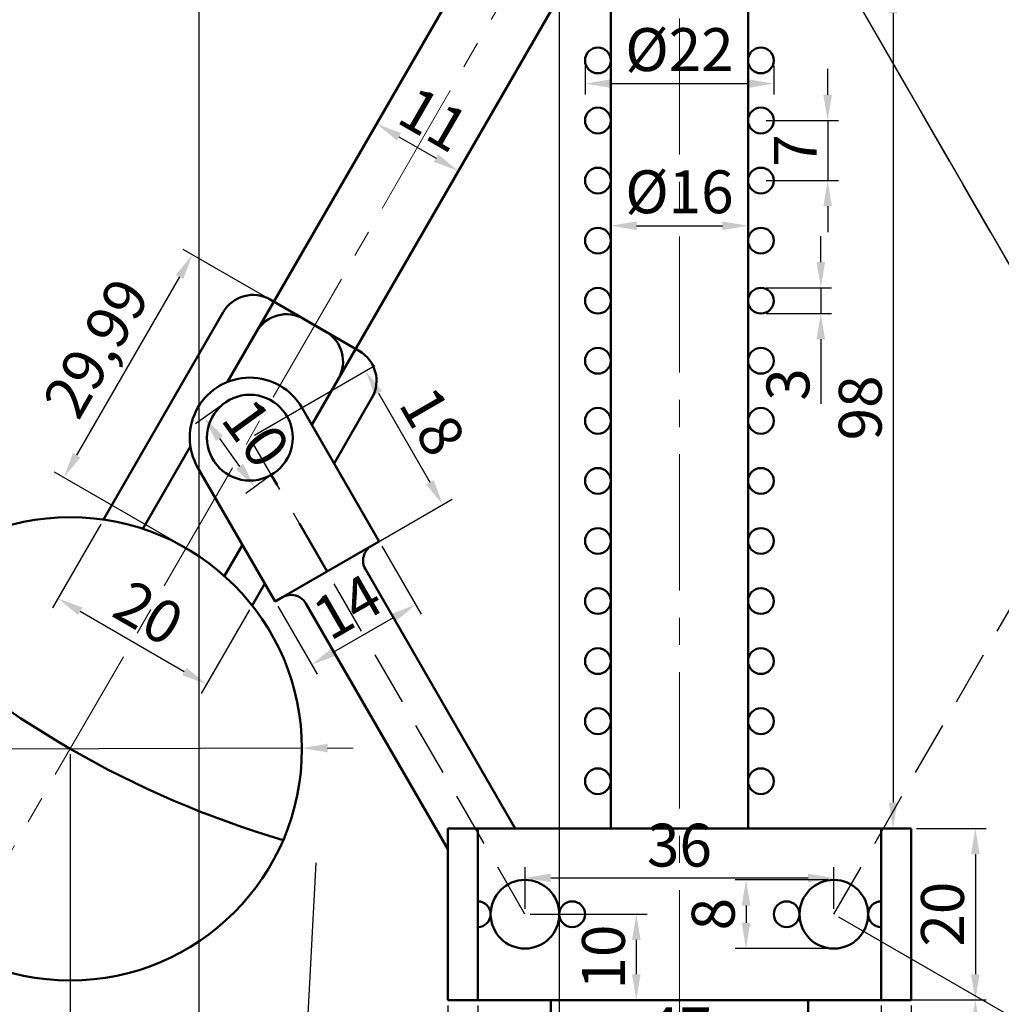
# Model space of a CAD drawing. Units: millimetres. Extents: x 98 to 674, y 38 to 476.
# Tile 4 of 7: x 200 to 315, y 197 to 312. Entities that reach past the tile are written whole.
import ezdxf

# ---------------------------------------------------------------- set-up
doc = ezdxf.new("R2010")
doc.units = ezdxf.units.MM
doc.header["$LTSCALE"] = 0.5
doc.linetypes.add('CENTER', pattern=[50.8, 31.75, -6.35, 6.35, -6.35])
doc.linetypes.add('DASHED', pattern=[19.05, 12.7, -6.35])
for name, color, linetype, lineweight in [('M-CNTR', 1, 'CENTER', 18), ('M-DIMS', 2, 'Continuous', 25), ('M-OUTL', 7, 'Continuous', 50), ('M-PHAN', 6, 'DASHED', 25)]:
    doc.layers.add(name, color=color, linetype=linetype, lineweight=lineweight)
doc.styles.get("Standard").update_dxf_attribs({"font": 'arial.ttf'})
doc.dimstyles.new('ISO-25', dxfattribs={"dimtxt": 5, "dimasz": 3, "dimexe": 1.25, "dimexo": 0.625, "dimtad": 1, "dimtxsty": 'Standard', "dimcen": 2.5, "dimadec": 0, "dimazin": 0, "dimtfac": 1, "dimtmove": 0, "dimatfit": 3, "dimfxl": 1, "dimarcsym": 0})

# ---------------------------------------------------------------- blocks, each defined once
blk = doc.blocks.new('*D17')
at = {"layer": 'Defpoints', "color": 0, "ltscale": 0.5, "transparency": 16777216}
for p in [(286.87, 300.19), (286.87, 293.19), (294.65, 293.19)]:
    blk.add_point(p, dxfattribs=at)
at = {"layer": 'M-DIMS', "color": 0, "lineweight": -2, "ltscale": 0.5, "transparency": 16777216}
for p, q in [((294.65, 303.19), (294.65, 306.19)), ((287.49, 300.19), (295.9, 300.19)), ((294.65, 300.19), (294.65, 293.19)), ((287.49, 293.19), (295.9, 293.19)), ((294.65, 290.19), (294.65, 287.19))]:
    blk.add_line(p, q, dxfattribs=at)
at = {"layer": 'M-DIMS', "color": 0, "ltscale": 0.5, "transparency": 16777216}
for points in [[(294.15, 303.19), (295.15, 303.19), (294.65, 300.19)], [(294.15, 290.19), (295.15, 290.19), (294.65, 293.19)]]:
    blk.add_solid(points, dxfattribs=at)
at = {"layer": 'M-DIMS', "color": 0, "ltscale": 0.5, "transparency": 16777216, "insert": (291.53, 296.69), "char_height": 5, "attachment_point": 5, "rotation": 90}
blk.add_mtext('7', dxfattribs=at)
blk = doc.blocks.new('*D18')
at = {"layer": 'Defpoints', "color": 0, "ltscale": 0.5, "transparency": 16777216}
for p in [(308.14, 315.69), (301.14, 217.69), (302.27, 217.69)]:
    blk.add_point(p, dxfattribs=at)
at = {"layer": 'M-DIMS', "color": 0, "lineweight": -2, "ltscale": 0.5, "transparency": 16777216}
for p, q in [((307.51, 315.69), (301.02, 315.69)), ((302.27, 312.69), (302.27, 220.69)), ((301.76, 217.69), (303.52, 217.69))]:
    blk.add_line(p, q, dxfattribs=at)
at = {"layer": 'M-DIMS', "color": 0, "ltscale": 0.5, "transparency": 16777216}
for points in [[(301.77, 312.69), (302.77, 312.69), (302.27, 315.69)], [(301.77, 220.69), (302.77, 220.69), (302.27, 217.69)]]:
    blk.add_solid(points, dxfattribs=at)
at = {"layer": 'M-DIMS', "color": 0, "ltscale": 0.5, "transparency": 16777216, "insert": (299.09, 266.69), "char_height": 5, "attachment_point": 5, "rotation": 90}
blk.add_mtext('98', dxfattribs=at)
blk = doc.blocks.new('*D19')
at = {"layer": 'Defpoints', "color": 0, "ltscale": 0.5, "transparency": 16777216}
for p in [(286.87, 280.69), (286.87, 277.69), (293.85, 277.69)]:
    blk.add_point(p, dxfattribs=at)
at = {"layer": 'M-DIMS', "color": 0, "lineweight": -2, "ltscale": 0.5, "transparency": 16777216}
for p, q in [((293.85, 283.69), (293.85, 286.69)), ((287.49, 280.69), (295.1, 280.69)), ((293.85, 280.69), (293.85, 277.69)), ((287.49, 277.69), (295.1, 277.69)), ((293.85, 274.69), (293.85, 267.16))]:
    blk.add_line(p, q, dxfattribs=at)
at = {"layer": 'M-DIMS', "color": 0, "ltscale": 0.5, "transparency": 16777216}
for points in [[(293.35, 283.69), (294.35, 283.69), (293.85, 280.69)], [(293.35, 274.69), (294.35, 274.69), (293.85, 277.69)]]:
    blk.add_solid(points, dxfattribs=at)
at = {"layer": 'M-DIMS', "color": 0, "ltscale": 0.5, "transparency": 16777216, "insert": (290.67, 269.42), "char_height": 5, "attachment_point": 5, "rotation": 90}
blk.add_mtext('3', dxfattribs=at)
blk = doc.blocks.new('*D20')
at = {"layer": 'Defpoints', "color": 0, "ltscale": 0.5, "transparency": 16777216}
for p in [(290.59, 325.69), (359.62, 281.36), (327.04, 262.55)]:
    blk.add_point(p, dxfattribs=at)
at = {"layer": 'M-DIMS', "color": 0, "lineweight": -2, "ltscale": 0.5, "transparency": 16777216}
for p, q in [((291.13, 326), (324.25, 345.12)), ((324.67, 341.9), (358.12, 283.96)), ((327.58, 262.86), (360.7, 281.99))]:
    blk.add_line(p, q, dxfattribs=at)
at = {"layer": 'M-DIMS', "color": 0, "ltscale": 0.5, "transparency": 16777216}
for points in [[(325.1, 342.15), (324.24, 341.65), (323.17, 344.5)], [(358.56, 284.21), (357.69, 283.71), (359.62, 281.36)]]:
    blk.add_solid(points, dxfattribs=at)
at = {"layer": 'M-DIMS', "color": 0, "ltscale": 0.5, "transparency": 16777216, "insert": (344.54, 314.74), "char_height": 5, "attachment_point": 5, "rotation": 300}
blk.add_mtext('72,9', dxfattribs=at)
blk = doc.blocks.new('*D21')
at = {"layer": 'Defpoints', "color": 0, "ltscale": 0.5, "transparency": 16777216}
for p in [(327.04, 262.55), (348.82, 249.98), (295.37, 207.69)]:
    blk.add_point(p, dxfattribs=at)
at = {"layer": 'M-DIMS', "color": 0, "lineweight": -2, "ltscale": 0.5, "transparency": 16777216}
for p, q in [((327.58, 262.24), (349.9, 249.35)), ((318.64, 197.71), (347.32, 247.38)), ((295.91, 207.37), (318.22, 194.49))]:
    blk.add_line(p, q, dxfattribs=at)
at = {"layer": 'M-DIMS', "color": 0, "ltscale": 0.5, "transparency": 16777216}
for points in [[(346.89, 247.63), (347.75, 247.13), (348.82, 249.98)], [(318.21, 197.96), (319.08, 197.46), (317.14, 195.11)]]:
    blk.add_solid(points, dxfattribs=at)
at = {"layer": 'M-DIMS', "color": 0, "ltscale": 0.5, "transparency": 16777216, "insert": (329.84, 224.36), "char_height": 5, "attachment_point": 5, "rotation": 60}
blk.add_mtext('63,35', dxfattribs=at)
blk = doc.blocks.new('*D22')
at = {"layer": 'Defpoints', "color": 0, "ltscale": 0.5, "transparency": 16777216}
for p in [(291.37, 325.69), (378.81, 252.55)]:
    blk.add_point(p, dxfattribs=at)
at = {"layer": 'M-DIMS', "color": 0, "lineweight": -2, "ltscale": 0.5, "transparency": 16777216}
blk.add_line((327.65, 295.34), (376.51, 254.47), dxfattribs=at)
blk.add_arc((291.37, 325.69), 114, 313.9161, 320.7202, dxfattribs=at)
at = {"layer": 'M-DIMS', "color": 0, "ltscale": 0.5, "transparency": 16777216}
blk.add_solid([(376.83, 254.86), (376.19, 254.09), (378.81, 252.55)], dxfattribs=at)
at = {"layer": 'M-DIMS', "color": 0, "ltscale": 0.5, "transparency": 16777216, "insert": (336.2, 292.27), "char_height": 5, "attachment_point": 5, "rotation": 320.0919}
blk.add_mtext('R114', dxfattribs=at)
blk = doc.blocks.new('*D23')
at = {"layer": 'Defpoints', "color": 0, "ltscale": 0.5, "transparency": 16777216}
for p in [(269.37, 288.95), (285.37, 288.95), (285.37, 287.92)]:
    blk.add_point(p, dxfattribs=at)
at = {"layer": 'M-DIMS', "color": 0, "lineweight": -2, "ltscale": 0.5, "transparency": 16777216}
for p, q in [((269.37, 288.33), (269.37, 286.67)), ((285.37, 288.33), (285.37, 286.67)), ((272.37, 287.92), (282.37, 287.92))]:
    blk.add_line(p, q, dxfattribs=at)
at = {"layer": 'M-DIMS', "color": 0, "ltscale": 0.5, "transparency": 16777216}
for points in [[(272.37, 288.42), (272.37, 287.42), (269.37, 287.92)], [(282.37, 288.42), (282.37, 287.42), (285.37, 287.92)]]:
    blk.add_solid(points, dxfattribs=at)
at = {"layer": 'M-DIMS', "color": 0, "ltscale": 0.5, "transparency": 16777216, "insert": (277.37, 291.23), "char_height": 5, "attachment_point": 5}
blk.add_mtext('%%C16', dxfattribs=at)
blk = doc.blocks.new('*D24')
at = {"layer": 'Defpoints', "color": 0, "ltscale": 0.5, "transparency": 16777216}
for p in [(266.37, 307.19), (288.37, 307.19), (288.37, 304.48)]:
    blk.add_point(p, dxfattribs=at)
at = {"layer": 'M-DIMS', "color": 0, "lineweight": -2, "ltscale": 0.5, "transparency": 16777216}
for p, q in [((266.37, 306.56), (266.37, 303.23)), ((288.37, 306.56), (288.37, 303.23)), ((269.37, 304.48), (285.37, 304.48))]:
    blk.add_line(p, q, dxfattribs=at)
at = {"layer": 'M-DIMS', "color": 0, "ltscale": 0.5, "transparency": 16777216}
for points in [[(269.37, 304.98), (269.37, 303.98), (266.37, 304.48)], [(285.37, 304.98), (285.37, 303.98), (288.37, 304.48)]]:
    blk.add_solid(points, dxfattribs=at)
at = {"layer": 'M-DIMS', "color": 0, "ltscale": 0.5, "transparency": 16777216, "insert": (277.37, 307.8), "char_height": 5, "attachment_point": 5}
blk.add_mtext('%%C22', dxfattribs=at)
blk = doc.blocks.new('*D25')
at = {"layer": 'Defpoints', "color": 0, "ltscale": 0.5, "transparency": 16777216}
for p in [(295.37, 211.91), (259.37, 207.69), (295.37, 207.69)]:
    blk.add_point(p, dxfattribs=at)
at = {"layer": 'M-DIMS', "color": 0, "lineweight": -2, "ltscale": 0.5, "transparency": 16777216}
for p, q in [((259.37, 208.31), (259.37, 213.16)), ((295.37, 208.31), (295.37, 213.16)), ((262.37, 211.91), (292.37, 211.91))]:
    blk.add_line(p, q, dxfattribs=at)
at = {"layer": 'M-DIMS', "color": 0, "ltscale": 0.5, "transparency": 16777216}
for points in [[(262.37, 212.41), (262.37, 211.41), (259.37, 211.91)], [(292.37, 212.41), (292.37, 211.41), (295.37, 211.91)]]:
    blk.add_solid(points, dxfattribs=at)
at = {"layer": 'M-DIMS', "color": 0, "ltscale": 0.5, "transparency": 16777216, "insert": (277.37, 215.09), "char_height": 5, "attachment_point": 5}
blk.add_mtext('36', dxfattribs=at)
blk = doc.blocks.new('*D26')
at = {"layer": 'Defpoints', "color": 0, "ltscale": 0.5, "transparency": 16777216}
for p in [(259.37, 207.69), (259.37, 197.69), (272.34, 197.69)]:
    blk.add_point(p, dxfattribs=at)
at = {"layer": 'M-DIMS', "color": 0, "lineweight": -2, "ltscale": 0.5, "transparency": 16777216}
for p, q in [((259.99, 207.69), (273.59, 207.69)), ((272.34, 204.69), (272.34, 200.69)), ((259.99, 197.69), (273.59, 197.69))]:
    blk.add_line(p, q, dxfattribs=at)
at = {"layer": 'M-DIMS', "color": 0, "ltscale": 0.5, "transparency": 16777216}
for points in [[(271.84, 204.69), (272.84, 204.69), (272.34, 207.69)], [(271.84, 200.69), (272.84, 200.69), (272.34, 197.69)]]:
    blk.add_solid(points, dxfattribs=at)
at = {"layer": 'M-DIMS', "color": 0, "ltscale": 0.5, "transparency": 16777216, "insert": (269.16, 202.69), "char_height": 5, "attachment_point": 5, "rotation": 90}
blk.add_mtext('10', dxfattribs=at)
blk = doc.blocks.new('*D27')
at = {"layer": 'Defpoints', "color": 0, "ltscale": 0.5, "transparency": 16777216}
for p in [(295.37, 211.69), (285.13, 203.69), (295.37, 203.69)]:
    blk.add_point(p, dxfattribs=at)
at = {"layer": 'M-DIMS', "color": 0, "lineweight": -2, "ltscale": 0.5, "transparency": 16777216}
for p, q in [((294.74, 211.69), (283.88, 211.69)), ((285.13, 208.69), (285.13, 206.69)), ((294.74, 203.69), (283.88, 203.69))]:
    blk.add_line(p, q, dxfattribs=at)
at = {"layer": 'M-DIMS', "color": 0, "ltscale": 0.5, "transparency": 16777216}
for points in [[(284.63, 208.69), (285.63, 208.69), (285.13, 211.69)], [(284.63, 206.69), (285.63, 206.69), (285.13, 203.69)]]:
    blk.add_solid(points, dxfattribs=at)
at = {"layer": 'M-DIMS', "color": 0, "ltscale": 0.5, "transparency": 16777216, "insert": (281.95, 207.69), "char_height": 5, "attachment_point": 5, "rotation": 90}
blk.add_mtext('8', dxfattribs=at)
blk = doc.blocks.new('*D28')
at = {"layer": 'Defpoints', "color": 0, "ltscale": 0.5, "transparency": 16777216}
for p in [(304.37, 217.69), (304.37, 197.69), (311.86, 197.69)]:
    blk.add_point(p, dxfattribs=at)
at = {"layer": 'M-DIMS', "color": 0, "lineweight": -2, "ltscale": 0.5, "transparency": 16777216}
for p, q in [((304.99, 217.69), (313.11, 217.69)), ((311.86, 214.69), (311.86, 200.69)), ((304.99, 197.69), (313.11, 197.69))]:
    blk.add_line(p, q, dxfattribs=at)
at = {"layer": 'M-DIMS', "color": 0, "ltscale": 0.5, "transparency": 16777216}
for points in [[(311.36, 214.69), (312.36, 214.69), (311.86, 217.69)], [(311.36, 200.69), (312.36, 200.69), (311.86, 197.69)]]:
    blk.add_solid(points, dxfattribs=at)
at = {"layer": 'M-DIMS', "color": 0, "ltscale": 0.5, "transparency": 16777216, "insert": (308.68, 207.69), "char_height": 5, "attachment_point": 5, "rotation": 90}
blk.add_mtext('20', dxfattribs=at)
blk = doc.blocks.new('*D29')
at = {"layer": 'Defpoints', "color": 0, "ltscale": 0.5, "transparency": 16777216}
for p in [(253.87, 197.69), (300.87, 197.69), (300.87, 190.55)]:
    blk.add_point(p, dxfattribs=at)
at = {"layer": 'M-DIMS', "color": 0, "lineweight": -2, "ltscale": 0.5, "transparency": 16777216}
for p, q in [((253.87, 197.06), (253.87, 189.3)), ((300.87, 197.06), (300.87, 189.3)), ((256.87, 190.55), (297.87, 190.55))]:
    blk.add_line(p, q, dxfattribs=at)
at = {"layer": 'M-DIMS', "color": 0, "ltscale": 0.5, "transparency": 16777216}
for points in [[(256.87, 191.05), (256.87, 190.05), (253.87, 190.55)], [(297.87, 191.05), (297.87, 190.05), (300.87, 190.55)]]:
    blk.add_solid(points, dxfattribs=at)
at = {"layer": 'M-DIMS', "color": 0, "ltscale": 0.5, "transparency": 16777216, "insert": (277.37, 193.67), "char_height": 5, "attachment_point": 5}
blk.add_mtext('47', dxfattribs=at)
blk = doc.blocks.new('*D30')
at = {"layer": 'Defpoints', "color": 0, "ltscale": 0.5, "transparency": 16777216}
for p in [(250.37, 197.69), (304.37, 197.69), (304.37, 183.26)]:
    blk.add_point(p, dxfattribs=at)
at = {"layer": 'M-DIMS', "color": 0, "lineweight": -2, "ltscale": 0.5, "transparency": 16777216}
for p, q in [((250.37, 197.06), (250.37, 182.01)), ((304.37, 197.06), (304.37, 182.01)), ((253.37, 183.26), (301.37, 183.26))]:
    blk.add_line(p, q, dxfattribs=at)
at = {"layer": 'M-DIMS', "color": 0, "ltscale": 0.5, "transparency": 16777216}
for points in [[(253.37, 183.76), (253.37, 182.76), (250.37, 183.26)], [(301.37, 183.76), (301.37, 182.76), (304.37, 183.26)]]:
    blk.add_solid(points, dxfattribs=at)
at = {"layer": 'M-DIMS', "color": 0, "ltscale": 0.5, "transparency": 16777216, "insert": (277.37, 186.43), "char_height": 5, "attachment_point": 5}
blk.add_mtext('54', dxfattribs=at)
blk = doc.blocks.new('*D33')
at = {"layer": 'Defpoints', "color": 0, "ltscale": 0.5, "transparency": 16777216}
for p in [(300.87, 197.69), (292.37, 177.69), (311.86, 177.69)]:
    blk.add_point(p, dxfattribs=at)
at = {"layer": 'M-DIMS', "color": 0, "lineweight": -2, "ltscale": 0.5, "transparency": 16777216}
for p, q in [((301.49, 197.69), (313.11, 197.69)), ((311.86, 194.69), (311.86, 180.69)), ((292.99, 177.69), (313.11, 177.69))]:
    blk.add_line(p, q, dxfattribs=at)
at = {"layer": 'M-DIMS', "color": 0, "ltscale": 0.5, "transparency": 16777216}
for points in [[(311.36, 194.69), (312.36, 194.69), (311.86, 197.69)], [(311.36, 180.69), (312.36, 180.69), (311.86, 177.69)]]:
    blk.add_solid(points, dxfattribs=at)
at = {"layer": 'M-DIMS', "color": 0, "ltscale": 0.5, "transparency": 16777216, "insert": (308.68, 187.69), "char_height": 5, "attachment_point": 5, "rotation": 90}
blk.add_mtext('20', dxfattribs=at)
blk = doc.blocks.new('*D60')
at = {"layer": 'Defpoints', "color": 0, "ltscale": 0.5, "transparency": 16777216}
for p in [(179.37, 226.88), (233.36, 227.04)]:
    blk.add_point(p, dxfattribs=at)
at = {"layer": 'M-DIMS', "color": 0, "lineweight": -2, "ltscale": 0.5, "transparency": 16777216}
for p, q in [((159.46, 226.81), (176.37, 226.87)), ((233.36, 227.04), (179.37, 226.88)), ((236.36, 227.05), (239.36, 227.06))]:
    blk.add_line(p, q, dxfattribs=at)
at = {"layer": 'M-DIMS', "color": 0, "ltscale": 0.5, "transparency": 16777216}
for points in [[(176.36, 227.37), (176.37, 226.37), (179.37, 226.88)], [(236.36, 227.55), (236.37, 226.55), (233.36, 227.04)]]:
    blk.add_solid(points, dxfattribs=at)
at = {"layer": 'M-DIMS', "color": 0, "ltscale": 0.5, "transparency": 16777216, "insert": (166.36, 230.15), "char_height": 5, "attachment_point": 5, "rotation": 0.1768}
blk.add_mtext('∅54', dxfattribs=at)
blk = doc.blocks.new('*D61')
at = {"layer": 'Defpoints', "color": 0, "ltscale": 0.5, "transparency": 16777216}
for p in [(210.24, 253.68), (227.57, 243.68), (222.26, 234.49)]:
    blk.add_point(p, dxfattribs=at)
at = {"layer": 'M-DIMS', "color": 0, "lineweight": -2, "ltscale": 0.5, "transparency": 16777216}
for p, q in [((209.93, 253.14), (204.31, 243.4)), ((207.54, 242.99), (219.66, 235.99)), ((227.25, 243.14), (221.63, 233.4))]:
    blk.add_line(p, q, dxfattribs=at)
at = {"layer": 'M-DIMS', "color": 0, "ltscale": 0.5, "transparency": 16777216}
for points in [[(207.79, 243.42), (207.29, 242.55), (204.94, 244.49)], [(219.91, 236.42), (219.41, 235.55), (222.26, 234.49)]]:
    blk.add_solid(points, dxfattribs=at)
at = {"layer": 'M-DIMS', "color": 0, "ltscale": 0.5, "transparency": 16777216, "insert": (215.19, 242.24), "char_height": 5, "attachment_point": 5, "rotation": 330}
blk.add_mtext('20', dxfattribs=at)
blk = doc.blocks.new('*D62')
at = {"layer": 'Defpoints', "color": 0, "ltscale": 0.5, "transparency": 16777216}
for p in [(242.36, 251.13), (230.24, 244.13), (246.63, 243.75)]:
    blk.add_point(p, dxfattribs=at)
at = {"layer": 'M-DIMS', "color": 0, "lineweight": -2, "ltscale": 0.5, "transparency": 16777216}
for p, q in [((242.68, 250.59), (247.25, 242.67)), ((230.55, 243.59), (235.13, 235.67)), ((237.1, 238.25), (244.03, 242.25))]:
    blk.add_line(p, q, dxfattribs=at)
at = {"layer": 'M-DIMS', "color": 0, "ltscale": 0.5, "transparency": 16777216}
for points in [[(243.78, 242.68), (244.28, 241.82), (246.63, 243.75)], [(236.85, 238.68), (237.35, 237.82), (234.5, 236.75)]]:
    blk.add_solid(points, dxfattribs=at)
at = {"layer": 'M-DIMS', "color": 0, "ltscale": 0.5, "transparency": 16777216, "insert": (239, 242.96), "char_height": 5, "attachment_point": 5, "rotation": 30}
blk.add_mtext('14', dxfattribs=at)
blk = doc.blocks.new('*D63')
at = {"layer": 'Defpoints', "color": 0, "ltscale": 0.5, "transparency": 16777216}
for p in [(227.3, 263.22), (249.79, 255.42), (236.3, 247.63)]:
    blk.add_point(p, dxfattribs=at)
at = {"layer": 'M-DIMS', "color": 0, "lineweight": -2, "ltscale": 0.5, "transparency": 16777216}
for p, q in [((227.84, 263.53), (241.87, 271.63)), ((242.29, 268.41), (248.29, 258.02)), ((236.84, 247.95), (250.87, 256.04))]:
    blk.add_line(p, q, dxfattribs=at)
at = {"layer": 'M-DIMS', "color": 0, "ltscale": 0.5, "transparency": 16777216}
for points in [[(242.72, 268.66), (241.85, 268.16), (240.79, 271.01)], [(248.72, 258.27), (247.85, 257.77), (249.79, 255.42)]]:
    blk.add_solid(points, dxfattribs=at)
at = {"layer": 'M-DIMS', "color": 0, "ltscale": 0.5, "transparency": 16777216, "insert": (248.04, 264.8), "char_height": 5, "attachment_point": 5, "rotation": 300}
blk.add_mtext('18', dxfattribs=at)
blk = doc.blocks.new('*D64')
at = {"layer": 'Defpoints', "color": 0, "ltscale": 0.5, "transparency": 16777216}
for p in [(224.37, 267.27), (230.23, 259.17), (227.86, 257.45)]:
    blk.add_point(p, dxfattribs=at)
at = {"layer": 'M-DIMS', "color": 0, "lineweight": -2, "ltscale": 0.5, "transparency": 16777216}
for p, q in [((223.87, 266.91), (220.98, 264.82)), ((223.76, 263.13), (226.1, 259.88)), ((229.72, 258.8), (226.84, 256.72))]:
    blk.add_line(p, q, dxfattribs=at)
at = {"layer": 'M-DIMS', "color": 0, "ltscale": 0.5, "transparency": 16777216}
for points in [[(224.16, 263.42), (223.35, 262.83), (222, 265.56)], [(226.5, 260.18), (225.69, 259.59), (227.86, 257.45)]]:
    blk.add_solid(points, dxfattribs=at)
at = {"layer": 'M-DIMS', "color": 0, "ltscale": 0.5, "transparency": 16777216, "insert": (227.5, 263.37), "char_height": 5, "attachment_point": 5, "rotation": 305.8717}
blk.add_mtext('10', dxfattribs=at)
blk = doc.blocks.new('*D65')
at = {"layer": 'Defpoints', "color": 0, "ltscale": 0.5, "transparency": 16777216}
for p in [(235.01, 276.23), (205.61, 258.57), (220.01, 250.26)]:
    blk.add_point(p, dxfattribs=at)
at = {"layer": 'M-DIMS', "color": 0, "lineweight": -2, "ltscale": 0.5, "transparency": 16777216}
for p, q in [((234.46, 276.55), (219.53, 285.17)), ((219.11, 281.95), (207.11, 261.17)), ((219.47, 250.57), (204.53, 259.19))]:
    blk.add_line(p, q, dxfattribs=at)
at = {"layer": 'M-DIMS', "color": 0, "ltscale": 0.5, "transparency": 16777216}
for points in [[(218.68, 282.2), (219.54, 281.7), (220.61, 284.54)], [(206.68, 261.42), (207.55, 260.92), (205.61, 258.57)]]:
    blk.add_solid(points, dxfattribs=at)
at = {"layer": 'M-DIMS', "color": 0, "ltscale": 0.5, "transparency": 16777216, "insert": (209.97, 273.37), "char_height": 5, "attachment_point": 5, "rotation": 60}
blk.add_mtext('29,99', dxfattribs=at)
blk = doc.blocks.new('*D66')
at = {"layer": 'Defpoints', "color": 0, "ltscale": 0.5, "transparency": 16777216}
for p in [(242.07, 299.8), (251.6, 294.3), (251.6, 294.3)]:
    blk.add_point(p, dxfattribs=at)
at = {"layer": 'M-DIMS', "color": 0, "lineweight": -2, "ltscale": 0.5, "transparency": 16777216}
for p, q in [((242.38, 300.34), (242.69, 300.88)), ((244.67, 298.3), (249, 295.8)), ((251.91, 294.84), (252.22, 295.38))]:
    blk.add_line(p, q, dxfattribs=at)
at = {"layer": 'M-DIMS', "color": 0, "ltscale": 0.5, "transparency": 16777216}
for points in [[(244.92, 298.73), (244.42, 297.87), (242.07, 299.8)], [(249.25, 296.23), (248.75, 295.37), (251.6, 294.3)]]:
    blk.add_solid(points, dxfattribs=at)
at = {"layer": 'M-DIMS', "color": 0, "ltscale": 0.5, "transparency": 16777216, "insert": (248.4, 299.77), "char_height": 5, "attachment_point": 5, "rotation": 330}
blk.add_mtext('11', dxfattribs=at)
blk = doc.blocks.new('BALL')
blk.add_circle((27, 27), 27)
blk.add_arc((84, 125.73), 114, 226.398, 253.602)
blk = doc.blocks.new('*D68')
at = {"layer": 'Defpoints', "color": 0, "ltscale": 0.5, "transparency": 16777216}
for p in [(263.37, 325.69), (206.37, 226.96), (263.37, 42.76)]:
    blk.add_point(p, dxfattribs=at)
at = {"layer": 'M-DIMS', "color": 0, "lineweight": -2, "ltscale": 0.5, "transparency": 16777216}
for p, q in [((263.37, 325.06), (263.37, 41.51)), ((206.37, 226.33), (206.37, 41.51)), ((209.37, 42.76), (260.37, 42.76))]:
    blk.add_line(p, q, dxfattribs=at)
at = {"layer": 'M-DIMS', "color": 0, "ltscale": 0.5, "transparency": 16777216}
for points in [[(209.37, 43.26), (209.37, 42.26), (206.37, 42.76)], [(260.37, 43.26), (260.37, 42.26), (263.37, 42.76)]]:
    blk.add_solid(points, dxfattribs=at)
at = {"layer": 'M-DIMS', "color": 0, "ltscale": 0.5, "transparency": 16777216, "insert": (234.87, 45.93), "char_height": 5, "attachment_point": 5}
blk.add_mtext('57', dxfattribs=at)
blk = doc.blocks.new('*D71')
at = {"layer": 'Defpoints', "color": 0, "ltscale": 0.5, "transparency": 16777216}
for p in [(269.37, 413.69), (121.37, 76.69), (269.37, 76.69)]:
    blk.add_point(p, dxfattribs=at)
at = {"layer": 'M-DIMS', "color": 0, "lineweight": -2, "ltscale": 0.5, "transparency": 16777216}
for p, q in [((268.74, 413.69), (120.12, 413.69)), ((121.37, 410.69), (121.37, 79.69)), ((268.74, 76.69), (120.12, 76.69))]:
    blk.add_line(p, q, dxfattribs=at)
at = {"layer": 'M-DIMS', "color": 0, "ltscale": 0.5, "transparency": 16777216}
for points in [[(120.87, 410.69), (121.87, 410.69), (121.37, 413.69)], [(120.87, 79.69), (121.87, 79.69), (121.37, 76.69)]]:
    blk.add_solid(points, dxfattribs=at)
at = {"layer": 'M-DIMS', "color": 0, "ltscale": 0.5, "transparency": 16777216, "insert": (118.19, 245.19), "char_height": 5, "attachment_point": 5, "rotation": 90}
blk.add_mtext('337', dxfattribs=at)
blk = doc.blocks.new('*D73')
at = {"layer": 'Defpoints', "color": 0, "ltscale": 0.5, "transparency": 16777216}
for p in [(221.4, 441.69), (221.4, 168.51), (149.37, 153.69)]:
    blk.add_point(p, dxfattribs=at)
at = {"layer": 'M-DIMS', "color": 0, "lineweight": -2, "ltscale": 0.5, "transparency": 16777216}
for p, q in [((149.37, 154.31), (149.37, 442.94)), ((221.4, 169.14), (221.4, 442.94)), ((152.37, 441.69), (218.4, 441.69))]:
    blk.add_line(p, q, dxfattribs=at)
at = {"layer": 'M-DIMS', "color": 0, "ltscale": 0.5, "transparency": 16777216}
for points in [[(152.37, 442.19), (152.37, 441.19), (149.37, 441.69)], [(218.4, 442.19), (218.4, 441.19), (221.4, 441.69)]]:
    blk.add_solid(points, dxfattribs=at)
at = {"layer": 'M-DIMS', "color": 0, "ltscale": 0.5, "transparency": 16777216, "insert": (185.38, 444.87), "char_height": 5, "attachment_point": 5}
blk.add_mtext('72.03', dxfattribs=at)
blk = doc.blocks.new('*D76')
at = {"layer": 'Defpoints', "color": 0, "ltscale": 0.5, "transparency": 16777216}
for p in [(234.98, 213.69), (230.99, 138.79)]:
    blk.add_point(p, dxfattribs=at)
at = {"layer": 'M-DIMS', "color": 0, "lineweight": -2, "ltscale": 0.5, "transparency": 16777216}
for p, q in [((234.98, 213.69), (230.99, 138.79)), ((228.25, 87.25), (230.84, 135.8))]:
    blk.add_line(p, q, dxfattribs=at)
at = {"layer": 'M-DIMS', "color": 0, "ltscale": 0.5, "transparency": 16777216}
blk.add_solid([(230.34, 135.82), (231.33, 135.77), (230.99, 138.79)], dxfattribs=at)
at = {"layer": 'M-DIMS', "color": 0, "ltscale": 0.5, "transparency": 16777216, "insert": (225.44, 94.02), "char_height": 5, "attachment_point": 5, "rotation": 86.9505}
blk.add_mtext('R75', dxfattribs=at)
blk = doc.blocks.new('*D78')
at = {"layer": 'Defpoints', "color": 0, "ltscale": 0.5, "transparency": 16777216}
for p in [(291.37, 325.69), (348.37, 226.96)]:
    blk.add_point(p, dxfattribs=at)
at = {"layer": 'M-DIMS', "color": 0, "lineweight": -2, "ltscale": 0.5, "transparency": 16777216}
for p, q in [((291.37, 325.69), (348.37, 226.96)), ((386.83, 160.33), (349.87, 224.36))]:
    blk.add_line(p, q, dxfattribs=at)
at = {"layer": 'M-DIMS', "color": 0, "ltscale": 0.5, "transparency": 16777216}
blk.add_solid([(350.3, 224.61), (349.43, 224.11), (348.37, 226.96)], dxfattribs=at)
at = {"layer": 'M-DIMS', "color": 0, "ltscale": 0.5, "transparency": 16777216, "insert": (385.28, 169.29), "char_height": 5, "attachment_point": 5, "rotation": 300.0001}
blk.add_mtext('R114', dxfattribs=at)

msp = doc.modelspace()

# ---------------------------------------------------------------- linework, layer by layer
at = {"layer": 'M-CNTR'}
for p, q in [((277.365, 413.6855), (277.365, 70.7639)), ((263.365, 325.6855), (192.865, 203.5759))]:
    msp.add_line(p, q, dxfattribs=at)
at = {"layer": 'M-OUTL'}
for p, q in [((251.2407, 315.6855), (224.7033, 269.7214)), ((263.9424, 315.6855), (234.5182, 264.7214)), ((269.365, 217.6855), (269.365, 315.6855)), ((285.365, 315.6855), (285.365, 217.6855)), ((220.3732, 262.2214), (214.8188, 252.601)), ((226.4353, 250.7214), (224.3451, 247.101)), ((250.365, 217.6855), (250.365, 197.6855)), ((304.365, 217.6855), (250.365, 217.6855)), ((253.865, 217.6855), (253.865, 197.6855)), ((285.365, 217.6855), (269.365, 217.6855)), ((300.865, 197.6855), (300.865, 217.6855)), ((304.365, 197.6855), (304.365, 217.6855)), ((250.365, 197.6855), (304.365, 197.6855)), ((292.365, 197.6855), (262.365, 197.6855)), ((262.365, 197.6855), (262.365, 177.6855)), ((292.365, 177.6855), (292.365, 197.6855))]:
    msp.add_line(p, q, dxfattribs=at)
at = {"layer": 'M-OUTL', "ltscale": 0.7}
for p, q in [((240.3431, 273.1432), (229.6689, 279.322)), ((224.2048, 277.8579), (210.2447, 253.6784)), ((236.1641, 275.572), (233.566, 277.072)), ((237.1163, 260.2214), (241.5253, 267.8579)), ((233.3635, 266.7214), (242.3635, 251.1329)), ((221.2392, 259.7214), (230.2392, 244.1329)), ((229.8014, 258.8913), (230.4768, 257.7214)), ((233.0749, 253.2214), (236.3014, 247.6329)), ((241.4975, 250.6329), (242.3635, 251.1329)), ((227.5652, 243.6784), (229.0334, 246.2214)), ((231.1052, 244.6329), (230.2392, 244.1329))]:
    msp.add_line(p, q, dxfattribs=at)
at = {"layer": 'M-OUTL', "ltscale": 0.5}
for p, q in [((231.1052, 244.6329), (241.4975, 250.6329)), ((240.7655, 247.9009), (258.2103, 217.6855)), ((233.8373, 243.9009), (250.365, 215.2739))]:
    msp.add_line(p, q, dxfattribs=at)
at = {"layer": 'M-OUTL'}
for centre, radius in [((267.865, 307.1855), 1.5), ((286.865, 307.1855), 1.5), ((267.865, 300.1855), 1.5), ((286.865, 300.1855), 1.5), ((267.865, 293.1855), 1.5), ((286.865, 293.1855), 1.5), ((267.865, 286.1855), 1.5), ((286.865, 286.1855), 1.5), ((267.865, 279.1855), 1.5), ((286.865, 279.1855), 1.5), ((267.865, 272.1855), 1.5), ((286.865, 272.1855), 1.5), ((267.865, 265.1855), 1.5), ((286.865, 265.1855), 1.5), ((267.865, 258.1855), 1.5), ((286.865, 258.1855), 1.5), ((267.865, 251.1855), 1.5), ((286.865, 251.1855), 1.5), ((267.865, 244.1855), 1.5), ((286.865, 244.1855), 1.5), ((267.865, 237.1855), 1.5), ((286.865, 237.1855), 1.5), ((267.865, 230.1855), 1.5), ((286.865, 230.1855), 1.5), ((267.865, 223.1855), 1.5), ((286.865, 223.1855), 1.5), ((259.365, 207.6855), 4), ((295.365, 207.6855), 4), ((264.865, 207.6855), 1.5), ((289.865, 207.6855), 1.5)]:
    msp.add_circle(centre, radius, dxfattribs=at)
at = {"layer": 'M-OUTL', "ltscale": 0.7}
msp.add_circle((227.3014, 263.2214), 5, dxfattribs=at)
for centre, radius, start, end in [((227.6689, 275.8579), 4, 60, 150), ((231.566, 273.6079), 4, 60, 150), ((234.1641, 272.1079), 4, 330, 60), ((238.0612, 269.8579), 4, 330, 60), ((227.3014, 263.2214), 7, 30, 210)]:
    msp.add_arc(centre, radius, start, end, dxfattribs=at)
at = {"layer": 'M-OUTL', "ltscale": 0.5}
for centre, start, end in [((242.4975, 248.9009), 120, 210), ((232.1052, 242.9009), 30, 120)]:
    msp.add_arc(centre, 2, start, end, dxfattribs=at)
at = {"layer": 'M-OUTL'}
for centre, start, end in [((253.865, 207.6855), 270, 90), ((300.865, 207.6855), 90, 270)]:
    msp.add_arc(centre, 1.5, start, end, dxfattribs=at)
at = {"layer": 'M-PHAN'}
for p, q in [((291.365, 325.6855), (375.7053, 179.6039)), ((259.365, 207.6855), (227.3014, 263.2214)), ((295.365, 207.6855), (327.4287, 263.2214))]:
    msp.add_line(p, q, dxfattribs=at)

# ---------------------------------------------------------------- block references
at = {"layer": 'M-OUTL'}
msp.add_blockref('BALL', (179.365, 199.959), dxfattribs=at)

# ---------------------------------------------------------------- dimensions: what is measured, and where the dimension line sits
at = {"layer": 'M-DIMS', "ltscale": 0.5}
for base, p1, p2, override, picture, middle in [((221.3997, 441.6855), (149.365, 153.6855), (221.3997, 168.5142), {"dimdec": 2, "dimlfac": 1, "dimrnd": 0, "dimzin": 0, "dimdsep": 46, "dimlunit": 2}, '*D73', (185.3824, 444.8651)), ((263.365, 42.7639), (206.365, 226.9586), (263.365, 325.6855), {"dimdec": 0, "dimlfac": 1, "dimrnd": 0, "dimzin": 0, "dimdsep": 46, "dimlunit": 2}, '*D68', (234.865, 45.9316)), ((304.365, 183.2593), (250.365, 197.6855), (304.365, 197.6855), {"dimclrd": 0, "dimclre": 0, "dimclrt": 0}, '*D30', (277.365, 186.4269)), ((300.865, 190.5497), (253.865, 197.6855), (300.865, 197.6855), {"dimclrd": 0, "dimclre": 0, "dimclrt": 0}, '*D29', (277.365, 193.6747))]:
    dim = msp.add_linear_dim(base=base, p1=p1, p2=p2, dimstyle='ISO-25', override=override, dxfattribs=at)
    dim.commit()
    dim.dimension.update_dxf_attribs({"geometry": picture, "text_midpoint": middle})
for base, p1, p2, override, picture, middle in [((121.365, 76.6855), (269.365, 413.6855), (269.365, 76.6855), {"dimdec": 0, "dimlfac": 1, "dimrnd": 0, "dimzin": 0, "dimdsep": 46, "dimlunit": 2}, '*D71', (118.1855, 245.1855)), ((302.2723, 217.6855), (308.1395, 315.6855), (301.1385, 217.6855), {"dimclrd": 0, "dimclre": 0, "dimclrt": 0}, '*D18', (299.0945, 266.6855)), ((294.6507, 293.1855), (286.865, 300.1855), (286.865, 293.1855), {"dimclrd": 0, "dimclre": 0, "dimclrt": 0}, '*D17', (291.5257, 296.6855)), ((293.8462, 277.6855), (286.865, 280.6855), (286.865, 277.6855), {"dimclrd": 0, "dimclre": 0, "dimclrt": 0}, '*D19', (290.6666, 269.4234)), ((311.8607, 197.6855), (304.365, 217.6855), (304.365, 197.6855), {"dimclrd": 0, "dimclre": 0, "dimclrt": 0}, '*D28', (308.6828, 207.6855)), ((285.1284, 203.6855), (295.365, 211.6855), (295.365, 203.6855), {"dimclrd": 0, "dimclre": 0, "dimclrt": 0}, '*D27', (281.9506, 207.6855)), ((272.3374, 197.6855), (259.365, 207.6855), (259.365, 197.6855), {"dimclrd": 0, "dimclre": 0, "dimclrt": 0}, '*D26', (269.1596, 202.6855)), ((311.8607, 177.6855), (300.865, 197.6855), (292.365, 177.6855), {"dimclrd": 0, "dimclre": 0, "dimclrt": 0}, '*D33', (308.6828, 187.6855))]:
    dim = msp.add_linear_dim(base=base, p1=p1, p2=p2, angle=90, dimstyle='ISO-25', override=override, dxfattribs=at)
    dim.commit()
    dim.dimension.update_dxf_attribs({"geometry": picture, "text_midpoint": middle})
for p1, p2, distance, picture, middle in [((290.5915, 325.6855), (327.0419, 262.5515), 37.6203, '*D20', (344.5403, 314.7435)), ((242.0694, 299.8004), (251.5957, 294.3004), 0, '*D66', (248.4002, 299.7656)), ((235.006, 276.2326), (220.0092, 250.2574), -16.6225, '*D65', (209.9686, 273.3712)), ((227.3014, 263.2214), (236.3014, 247.6329), 15.5705, '*D63', (248.038, 264.8014)), ((224.3715, 267.273), (230.2312, 259.1697), -2.9299, '*D64', (227.5023, 263.3667)), ((295.365, 207.6855), (327.0419, 262.5515), -25.146, '*D21', (329.8371, 224.3604)), ((210.2447, 253.6784), (227.5652, 243.6784), -10.6153, '*D61', (215.1863, 242.2374)), ((230.2392, 244.1329), (242.3635, 251.1329), -8.5255, '*D62', (238.9965, 242.9648))]:
    dim = msp.add_aligned_dim(p1=p1, p2=p2, distance=distance, dimstyle='ISO-25', override={"dimclrd": 0, "dimclre": 0, "dimclrt": 0}, dxfattribs=at)
    dim.commit()
    dim.dimension.update_dxf_attribs({"geometry": picture, "text_midpoint": middle})
for center, mpoint, override, picture, middle in [((291.365, 325.6855), (378.8115, 252.5479), {"dimclrd": 0, "dimclre": 0, "dimclrt": 0}, '*D22', (334.1894, 289.8685)), ((291.365, 325.6855), (348.3652, 226.9587), {"dimdec": 0, "dimlfac": 1, "dimrnd": 0, "dimzin": 0, "dimdsep": 46, "dimlunit": 2}, '*D78', (382.5653, 167.7226)), ((234.9849, 213.6855), (230.995, 138.7917), {"dimdec": 0, "dimlfac": 1, "dimrnd": 0, "dimzin": 0, "dimdsep": 46, "dimlunit": 2}, '*D76', (228.601, 93.8554))]:
    dim = msp.add_radius_dim(center=center, mpoint=mpoint, dimstyle='ISO-25', override=override, dxfattribs=at)
    dim.commit()
    dim.dimension.update_dxf_attribs({"geometry": picture, "text_midpoint": middle, "dimtype": 164})
for base, p1, p2, picture, middle in [((288.365, 304.4839), (266.365, 307.1855), (288.365, 307.1855), '*D24', (277.365, 307.8016)), ((285.365, 287.9168), (269.365, 288.9502), (285.365, 288.9502), '*D23', (277.365, 291.2345))]:
    dim = msp.add_linear_dim(base=base, p1=p1, p2=p2, text='%%C<>', dimstyle='ISO-25', override={"dimclrd": 0, "dimclre": 0, "dimclrt": 0}, dxfattribs=at)
    dim.commit()
    dim.dimension.update_dxf_attribs({"geometry": picture, "text_midpoint": middle})
dim = msp.add_diameter_dim_2p(p1=(233.3649, 227.0419), p2=(179.3652, 226.8753), dimstyle='ISO-25', override={"dimclrd": 0, "dimclre": 0, "dimclrt": 0}, dxfattribs=at)
dim.commit()
dim.dimension.update_dxf_attribs({"geometry": '*D60', "text_midpoint": (166.3749, 226.8352), "dimtype": 163})
dim = msp.add_linear_dim(base=(295.365, 211.9103), p1=(259.365, 207.6855), p2=(295.365, 207.6855), dimstyle='ISO-25', override={"dimclrd": 0, "dimclre": 0, "dimclrt": 0}, dxfattribs=at)
dim.commit()
dim.dimension.update_dxf_attribs({"geometry": '*D25', "text_midpoint": (277.365, 211.9103), "dimtype": 160})

doc.saveas('drawing.dxf')
